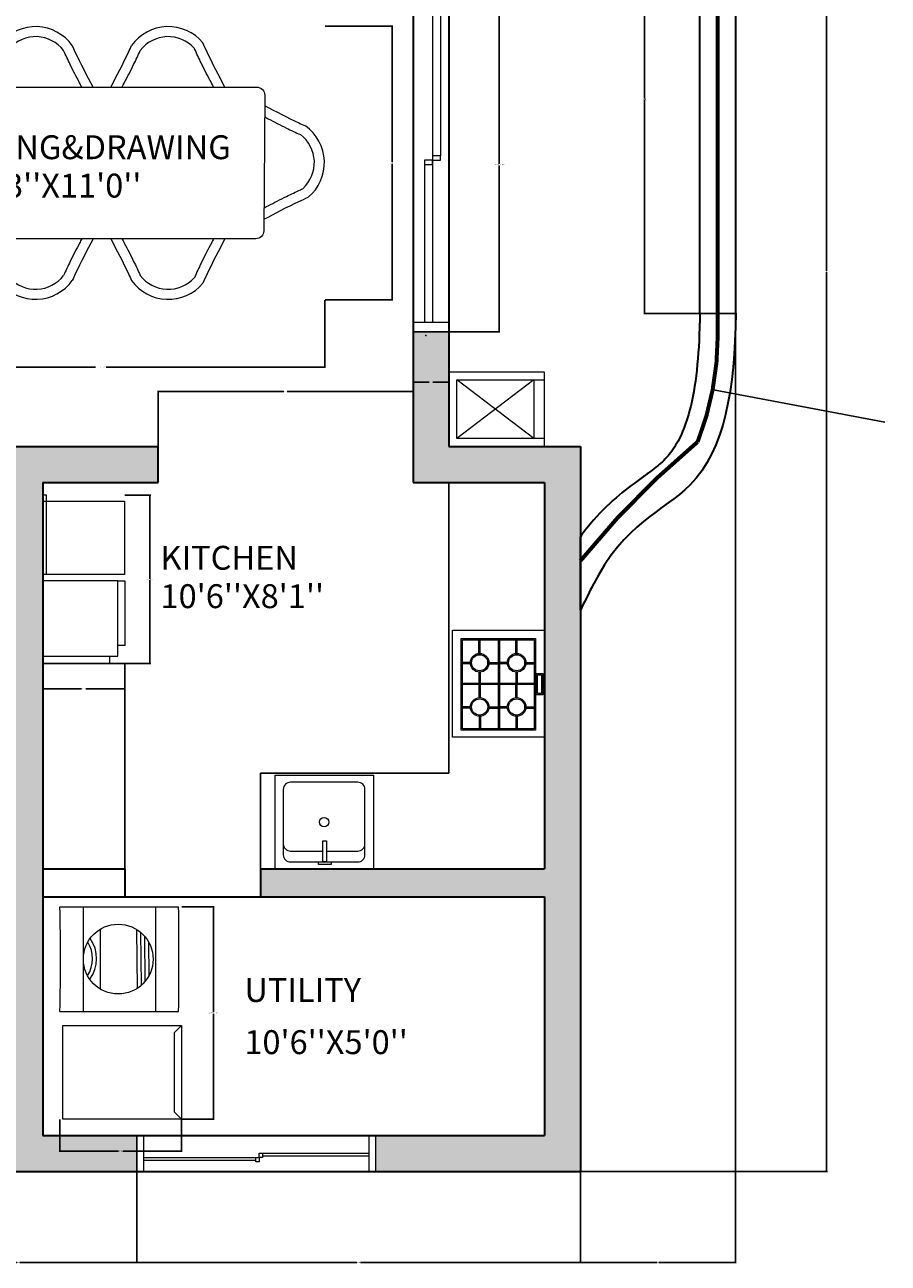
# Model space of a CAD drawing. Units: inches. Extents: x 1789 to 2841, y 3180 to 3702.
# Tile 11 of 14: x 2624 to 2841, y 3180 to 3491. Entities that reach past the tile are written whole.
import ezdxf

# ---------------------------------------------------------------- set-up
doc = ezdxf.new("R2010")
doc.units = ezdxf.units.IN
doc.header["$MEASUREMENT"] = 0
for name, color, linetype, lineweight in [('A-ANNO-DIMS', 2, 'Continuous', 18), ('A-AREA-IDEN', 7, 'Continuous', 18), ('A-EQPM', 8, 'Continuous', 18), ('A-FLOR-CASE', 34, 'Continuous', 25), ('A-FLOR-FIXT', 9, 'Continuous', 18), ('A-FLOR-HRAL', 40, 'Continuous', 18), ('A-WALL', 40, 'Continuous', 35), ('A-WALL-PATT', 252, 'Continuous', 13), ('FURNITURE', 34, 'Continuous', 18), ('WINDOWS', 130, 'Continuous', 18)]:
    doc.layers.add(name, color=color, linetype=linetype, lineweight=lineweight)
doc.styles.get("Standard").update_dxf_attribs({"font": 'arial.ttf'})
doc.dimstyles.get("Standard").update_dxf_attribs({"dimtxt": 0.18, "dimasz": 0.18, "dimexe": 0.18, "dimexo": 0.0625, "dimgap": 0.09, "dimtad": 0, "dimtih": 1, "dimtoh": 1, "dimdec": 0, "dimzin": 0, "dimdsep": 46, "dimlunit": 3, "dimtxsty": 'Standard', "dimcen": 0.09, "dimadec": 0, "dimazin": 0, "dimtfac": 1, "dimtdec": 0, "dimtofl": 0, "dimtmove": 0, "dimatfit": 3, "dimfxl": 1, "dimtolj": 1, "dimtzin": 0, "dimarcsym": 0})

# ---------------------------------------------------------------- blocks, each defined once
blk = doc.blocks.new('WINDOW')
for p, q in [((1997.14, 3495.61), (1997.14, 3458.2)), ((1999.14, 3495.61), (1999.14, 3458.2)), ((1995.14, 3457.08), (1995.14, 3416.32)), ((1997.14, 3457.08), (1997.14, 3416.32))]:
    blk.add_line(p, q)
for points in [[(1992.23, 3497.95), (2001.23, 3497.95), (2001.23, 3413.99), (1992.23, 3413.99)], [(1992.23, 3497.95), (2001.23, 3497.95), (2001.23, 3495.61), (1992.23, 3495.61)], [(1997.14, 3457.08), (1999.14, 3457.08), (1999.14, 3458.2), (1997.14, 3458.2)], [(1995.14, 3455.97), (1997.14, 3455.97), (1997.14, 3457.08), (1995.14, 3457.08)], [(1992.23, 3413.99), (2001.23, 3413.99), (2001.23, 3416.32), (1992.23, 3416.32)]]:
    blk.add_lwpolyline(points, close=True)
blk = doc.blocks.new('HYJ')
for p, q in [((2236.02, 3650.77), (2262.74, 3650.77)), ((2206.12, 3649.67), (2234.3, 3649.67)), ((2206.12, 3649), (2234.3, 3649)), ((2236.02, 3650.11), (2262.74, 3650.11))]:
    blk.add_line(p, q)
for points in [[(2204.43, 3646.16), (2264.43, 3646.16), (2264.43, 3655.16), (2204.43, 3655.16)], [(2204.43, 3655.16), (2206.12, 3655.16), (2206.12, 3646.16), (2204.43, 3646.16)], [(2264.43, 3655.16), (2262.74, 3655.16), (2262.74, 3646.16), (2264.43, 3646.16)], [(2235.16, 3650.77), (2236.02, 3650.77), (2236.02, 3649.67), (2235.16, 3649.67)], [(2234.3, 3649.67), (2235.16, 3649.67), (2235.16, 3648.56), (2234.3, 3648.56)]]:
    blk.add_lwpolyline(points, close=True)
blk = doc.blocks.new('WASH')
for p, q in [((2194.57, 3269.63), (2224.37, 3269.63)), ((2200.44, 3243.35), (2200.44, 3269.63)), ((2218.58, 3269.63), (2218.58, 3243.35)), ((2204.7, 3264.01), (2204.68, 3248.99)), ((2213.79, 3263.95), (2213.93, 3249.12)), ((2214.8, 3263.23), (2214.92, 3249.86)), ((2215.81, 3262.24), (2215.91, 3250.86)), ((2216.82, 3260.81), (2216.9, 3252.31)), ((2194.57, 3243.35), (2224.37, 3243.35)), ((2225.07, 3239.8), (2223.31, 3238.03)), ((2223.31, 3218.04), (2223.31, 3238.03)), ((2225.07, 3216.27), (2223.31, 3218.04))]:
    blk.add_line(p, q)
blk.add_lwpolyline([(2195.28, 3239.8), (2225.07, 3239.8), (2225.07, 3216.27), (2195.28, 3216.27)], close=True)
blk.add_circle((2209.2, 3256.49), 8.76)
for centre, radius, start, end in [((1539.89, 3256.49), 654.81, 358.85012, 1.14988), ((1226.25, 3256.49), 998.2, 359.24572, 0.75428), ((2194.95, 3256.62), 7.81, 326.7676, 32.1994), ((2194.95, 3256.62), 8.81, 323.7828, 35.1842)]:
    blk.add_arc(centre, radius, start, end)
blk = doc.blocks.new('SINK')
for points in [[(2247.56, 3305.33), (2275.07, 3305.33), (2275.07, 3279.16), (2247.56, 3279.16)], [(2260.91, 3287.01), (2261.87, 3287.01), (2261.87, 3281.09), (2260.91, 3281.09)], [(2259.67, 3281.09), (2263.21, 3281.09), (2263.21, 3280.41), (2259.67, 3280.41)]]:
    blk.add_lwpolyline(points, close=True)
blk.add_lwpolyline([(2251.84, 3281.09), (2270.63, 3281.09, 0.414214), (2272.63, 3283.09), (2272.63, 3301.33, 0.414214), (2270.63, 3303.33), (2251.84, 3303.33, 0.414214), (2249.84, 3301.33), (2249.84, 3283.09, 0.414214)], format="xyb", close=True)
for points in [[(2249.84, 3301.33), (2249.84, 3286.11, 0.414214), (2251.84, 3284.11), (2260.91, 3284.11)], [(2261.87, 3284.11), (2270.63, 3284.11, 0.414214), (2272.63, 3286.11), (2272.63, 3301.33)]]:
    blk.add_lwpolyline(points, format="xyb")
blk.add_circle((2261.24, 3292.21), 1.3)
blk = doc.blocks.new('STOVE')
for p, q in [((2291.13, 3337.23), (2291.13, 3342.37)), ((2291.63, 3337.23), (2291.63, 3342.37)), ((2298.52, 3342.42), (2298.52, 3308.4)), ((2299.02, 3342.42), (2299.02, 3308.4)), ((2305.31, 3337.23), (2305.31, 3342.37)), ((2305.81, 3337.23), (2305.81, 3342.37)), ((2287.79, 3333.73), (2284.84, 3333.73)), ((2287.81, 3333.23), (2284.84, 3333.23)), ((2294.92, 3333.23), (2298.52, 3333.23)), ((2294.94, 3333.73), (2298.52, 3333.73)), ((2301.97, 3333.73), (2299.02, 3333.73)), ((2301.99, 3333.23), (2299.02, 3333.23)), ((2309.1, 3333.23), (2312.22, 3333.23)), ((2309.12, 3333.73), (2312.22, 3333.73)), ((2291.13, 3330.09), (2291.13, 3325.91)), ((2291.63, 3330.09), (2291.63, 3325.91)), ((2305.31, 3330.09), (2305.31, 3325.91)), ((2305.81, 3330.09), (2305.81, 3325.91)), ((2284.82, 3325.91), (2312.22, 3325.91)), ((2284.82, 3325.41), (2312.22, 3325.41)), ((2291.15, 3320.29), (2291.15, 3325.43)), ((2291.65, 3320.29), (2291.65, 3325.43)), ((2305.31, 3320.29), (2305.31, 3325.43)), ((2305.31, 3325.41), (2305.31, 3325.34)), ((2305.81, 3320.29), (2305.81, 3325.43)), ((2305.81, 3325.41), (2305.81, 3325.34)), ((2287.8, 3316.79), (2284.82, 3316.79)), ((2287.83, 3316.29), (2284.82, 3316.29)), ((2291.15, 3313.15), (2291.15, 3308.4)), ((2291.65, 3313.15), (2291.65, 3308.4)), ((2294.94, 3316.29), (2298.52, 3316.29)), ((2294.96, 3316.79), (2298.52, 3316.79)), ((2301.97, 3316.79), (2299.02, 3316.79)), ((2301.99, 3316.29), (2299.02, 3316.29)), ((2305.31, 3313.15), (2305.31, 3308.4)), ((2305.81, 3313.15), (2305.81, 3308.4)), ((2309.1, 3316.29), (2312.22, 3316.29)), ((2309.12, 3316.79), (2312.22, 3316.79))]:
    blk.add_line(p, q)
for points in [[(2280.96, 3346.14), (2316.23, 3346.14), (2316.23, 3305.13), (2280.96, 3305.13)], [(2284.32, 3342.92), (2312.72, 3342.92), (2312.72, 3307.9), (2284.32, 3307.9)], [(2284.82, 3342.42), (2312.22, 3342.42), (2312.22, 3308.4), (2284.82, 3308.4)], [(2313.05, 3329.49), (2315.55, 3329.49), (2315.55, 3321.33), (2313.05, 3321.33)], [(2313.55, 3328.99), (2315.05, 3328.99), (2315.05, 3321.83), (2313.55, 3321.83)]]:
    blk.add_lwpolyline(points, close=True)
for centre, radius in [((2291.37, 3333.66), 3.58), ((2291.37, 3333.66), 3.08), ((2305.55, 3333.66), 3.58), ((2305.55, 3333.66), 3.08), ((2291.38, 3316.72), 3.58), ((2291.38, 3316.72), 3.08), ((2305.55, 3316.72), 3.58), ((2305.55, 3316.72), 3.08)]:
    blk.add_circle(centre, radius)
blk = doc.blocks.new('BYY')
for p, q in [((2191.23, 3321.4), (2190.23, 3321.4)), ((2190.23, 3321.4), (2190.23, 3319.89)), ((2191.23, 3301.51), (2191.23, 3321.4)), ((2209.12, 3299.92), (2210.83, 3299.92)), ((2210.83, 3299.92), (2210.83, 3283.66)), ((2190.23, 3279.16), (2190.23, 3281.03)), ((2207.05, 3281.03), (2207.05, 3279.16)), ((2210.83, 3283.66), (2209.12, 3283.66)), ((2207.05, 3279.16), (2190.23, 3279.16))]:
    blk.add_line(p, q)
for points in [[(2190.23, 3319.89), (2210.75, 3319.89), (2210.75, 3301.51), (2190.23, 3301.51)], [(2190.23, 3281.03), (2209.12, 3281.03), (2209.12, 3299.92), (2190.23, 3299.92)]]:
    blk.add_lwpolyline(points, close=True)
blk = doc.blocks.new('DINI')
blk.add_lwpolyline([(2038.22, 3475.42), (2115.97, 3475.42, -0.414214), (2117.97, 3473.42), (2117.72, 3439.35, -0.414214), (2115.72, 3437.35), (2037.97, 3437.35, -0.414214), (2035.97, 3439.35), (2036.22, 3473.42, -0.414214)], format="xyb", close=True)
for centre, radius, start, end in [((2060.43, 3479.31), 11.31, 35.4017, 140.0736), ((2093.76, 3479.31), 11.31, 39.9264, 144.5983), ((2060.43, 3479.31), 8.8, 36.8657, 137.9611), ((2093.76, 3479.31), 8.8, 42.0389, 143.1343), ((2032.05, 3456.46), 11.31, 125.4017, 230.0736), ((2121.64, 3456.46), 11.31, 309.9264, 54.5983), ((2032.05, 3456.46), 8.8, 126.8657, 227.9611), ((2121.64, 3456.46), 8.8, 312.0389, 53.1343), ((2060.43, 3433.45), 11.31, 219.9264, 324.5983), ((2060.43, 3433.45), 8.8, 222.0389, 323.1343), ((2093.76, 3433.45), 11.31, 215.4017, 320.0736), ((2093.76, 3433.45), 8.8, 216.8657, 317.9611)]:
    blk.add_arc(centre, radius, start, end)
for points, knots in [([(2046.22, 3475.42), (2047.75, 3478.33), (2049.68, 3482.01), (2051.4, 3485.79), (2051.76, 3486.58)], [0, 0, 0, 0, 7.856931, 9.915256, 9.915256, 9.915256, 9.915256]), ([(2074.88, 3475.42), (2073.35, 3478.33), (2071.54, 3481.78), (2069.91, 3485.32), (2069.66, 3485.87)], [0, 0, 0, 0, 7.856931, 9.297576, 9.297576, 9.297576, 9.297576]), ([(2079.31, 3475.42), (2080.85, 3478.33), (2082.66, 3481.78), (2084.29, 3485.32), (2084.54, 3485.87)], [0, 0, 0, 0, 7.856931, 9.297576, 9.297576, 9.297576, 9.297576]), ([(2107.98, 3475.42), (2106.45, 3478.33), (2104.51, 3482.01), (2102.79, 3485.79), (2102.44, 3486.58)], [0, 0, 0, 0, 7.856931, 9.915256, 9.915256, 9.915256, 9.915256]), ([(2049.05, 3475.42), (2049.25, 3475.79), (2049.44, 3476.15), (2050.42, 3478.03), (2051.21, 3479.56), (2052.54, 3482.27), (2053.1, 3483.45), (2053.72, 3484.82), (2053.81, 3485.01), (2053.9, 3485.21)], [1.048693, 1.048693, 1.048693, 1.048693, 2.029233, 2.029233, 6.0877, 6.0877, 9.118148, 9.118148, 9.624349, 9.624349, 9.624349, 9.624349]), ([(2072.04, 3475.42), (2071.85, 3475.78), (2071.66, 3476.15), (2070.68, 3478.03), (2069.89, 3479.55), (2068.56, 3482.26), (2068.01, 3483.43), (2067.48, 3484.59)], [1.048889, 1.048889, 1.048889, 1.048889, 2.02655, 2.02655, 6.079649, 6.079649, 9.095857, 9.095857, 9.095857, 9.095857]), ([(2082.15, 3475.42), (2082.34, 3475.78), (2082.53, 3476.15), (2083.51, 3478.03), (2084.3, 3479.55), (2085.63, 3482.26), (2086.19, 3483.43), (2086.72, 3484.59)], [1.048889, 1.048889, 1.048889, 1.048889, 2.02655, 2.02655, 6.079649, 6.079649, 9.095857, 9.095857, 9.095857, 9.095857]), ([(2105.14, 3475.42), (2104.95, 3475.79), (2104.76, 3476.15), (2103.78, 3478.03), (2102.99, 3479.56), (2101.65, 3482.27), (2101.1, 3483.45), (2100.47, 3484.82), (2100.38, 3485.01), (2100.3, 3485.21)], [1.048693, 1.048693, 1.048693, 1.048693, 2.029233, 2.029233, 6.0877, 6.0877, 9.118148, 9.118148, 9.624349, 9.624349, 9.624349, 9.624349]), ([(2036.2, 3471.04), (2036.05, 3470.96), (2035.89, 3470.88), (2035.74, 3470.8), (2035.74, 3470.8), (2035.74, 3470.8), (2035.74, 3470.8), (2032.89, 3469.3), (2029.51, 3467.53), (2026.05, 3465.93), (2025.5, 3465.68)], [-0.229823, -0.229823, -0.229823, -0.229823, 0.189373, 0.189373, 0.189373, 0.189712, 0.189712, 0.189712, 7.856931, 9.297576, 9.297576, 9.297576, 9.297576]), ([(2117.95, 3470.8), (2120.8, 3469.3), (2124.18, 3467.53), (2127.64, 3465.93), (2128.19, 3465.68)], [0.189712, 0.189712, 0.189712, 0.189712, 7.856931, 9.297576, 9.297576, 9.297576, 9.297576]), ([(2036.18, 3468.19), (2036.04, 3468.12), (2035.9, 3468.04), (2035.76, 3467.97), (2035.76, 3467.97), (2035.76, 3467.97), (2035.76, 3467.97), (2035.46, 3467.81), (2035.16, 3467.65), (2033.34, 3466.71), (2031.81, 3465.92), (2029.11, 3464.59), (2027.94, 3464.04), (2026.77, 3463.5)], [0.838882, 0.838882, 0.838882, 0.838882, 1.215073, 1.215073, 1.215073, 1.219193, 1.219193, 1.219193, 2.02655, 2.02655, 6.079649, 6.079649, 9.095857, 9.095857, 9.095857, 9.095857]), ([(2117.93, 3467.97), (2118.23, 3467.81), (2118.53, 3467.65), (2120.35, 3466.71), (2121.88, 3465.92), (2124.58, 3464.59), (2125.75, 3464.04), (2126.92, 3463.5)], [1.219193, 1.219193, 1.219193, 1.219193, 2.02655, 2.02655, 6.079649, 6.079649, 9.095857, 9.095857, 9.095857, 9.095857]), ([(2035.95, 3445.08), (2035.58, 3445.27), (2035.22, 3445.46), (2033.34, 3446.45), (2031.81, 3447.23), (2029.1, 3448.57), (2027.92, 3449.12), (2026.55, 3449.75), (2026.36, 3449.84), (2026.16, 3449.93)], [1.048693, 1.048693, 1.048693, 1.048693, 2.029233, 2.029233, 6.0877, 6.0877, 9.118148, 9.118148, 9.624349, 9.624349, 9.624349, 9.624349]), ([(2117.74, 3445.08), (2118.11, 3445.27), (2118.47, 3445.46), (2120.35, 3446.45), (2121.88, 3447.23), (2124.59, 3448.57), (2125.77, 3449.12), (2127.14, 3449.75), (2127.33, 3449.84), (2127.53, 3449.93)], [1.048693, 1.048693, 1.048693, 1.048693, 2.029233, 2.029233, 6.0877, 6.0877, 9.118148, 9.118148, 9.624349, 9.624349, 9.624349, 9.624349]), ([(2035.95, 3442.24), (2033.03, 3443.77), (2029.36, 3445.71), (2025.58, 3447.43), (2024.79, 3447.79)], [0, 0, 0, 0, 7.856931, 9.915256, 9.915256, 9.915256, 9.915256]), ([(2117.74, 3442.24), (2120.66, 3443.77), (2124.33, 3445.71), (2128.11, 3447.43), (2128.9, 3447.79)], [0, 0, 0, 0, 7.856931, 9.915256, 9.915256, 9.915256, 9.915256]), ([(2046.22, 3437.35), (2047.75, 3434.43), (2049.68, 3430.75), (2051.4, 3426.98), (2051.76, 3426.19)], [0, 0, 0, 0, 7.856931, 9.915256, 9.915256, 9.915256, 9.915256]), ([(2049.05, 3437.35), (2049.25, 3436.98), (2049.44, 3436.62), (2050.42, 3434.73), (2051.21, 3433.2), (2052.54, 3430.5), (2053.1, 3429.32), (2053.72, 3427.95), (2053.81, 3427.75), (2053.9, 3427.56)], [1.048693, 1.048693, 1.048693, 1.048693, 2.029233, 2.029233, 6.0877, 6.0877, 9.118148, 9.118148, 9.624349, 9.624349, 9.624349, 9.624349]), ([(2072.04, 3437.35), (2071.85, 3436.98), (2071.66, 3436.62), (2070.68, 3434.74), (2069.89, 3433.21), (2068.56, 3430.51), (2068.01, 3429.34), (2067.48, 3428.17)], [1.048889, 1.048889, 1.048889, 1.048889, 2.02655, 2.02655, 6.079649, 6.079649, 9.095857, 9.095857, 9.095857, 9.095857]), ([(2074.88, 3437.35), (2073.35, 3434.43), (2071.54, 3430.98), (2069.91, 3427.45), (2069.66, 3426.9)], [0, 0, 0, 0, 7.856931, 9.297576, 9.297576, 9.297576, 9.297576]), ([(2079.31, 3437.35), (2080.85, 3434.43), (2082.66, 3430.98), (2084.29, 3427.45), (2084.54, 3426.9)], [0, 0, 0, 0, 7.856931, 9.297576, 9.297576, 9.297576, 9.297576]), ([(2082.15, 3437.35), (2082.34, 3436.98), (2082.53, 3436.62), (2083.51, 3434.74), (2084.3, 3433.21), (2085.63, 3430.51), (2086.19, 3429.34), (2086.72, 3428.17)], [1.048889, 1.048889, 1.048889, 1.048889, 2.02655, 2.02655, 6.079649, 6.079649, 9.095857, 9.095857, 9.095857, 9.095857]), ([(2105.14, 3437.35), (2104.95, 3436.98), (2104.76, 3436.62), (2103.78, 3434.73), (2102.99, 3433.2), (2101.65, 3430.5), (2101.1, 3429.32), (2100.47, 3427.95), (2100.38, 3427.75), (2100.3, 3427.56)], [1.048693, 1.048693, 1.048693, 1.048693, 2.029233, 2.029233, 6.0877, 6.0877, 9.118148, 9.118148, 9.624349, 9.624349, 9.624349, 9.624349]), ([(2107.98, 3437.35), (2106.45, 3434.43), (2104.51, 3430.75), (2102.79, 3426.98), (2102.44, 3426.19)], [0, 0, 0, 0, 7.856931, 9.915256, 9.915256, 9.915256, 9.915256])]:
    blk.add_open_spline(points, degree=3, knots=knots)
blk = doc.blocks.new('GTGTGTGT')
for p, q in [((1970.85, 3401.93), (1970.85, 3387.16)), ((1970.92, 3401.93), (1990.23, 3387.16)), ((1970.92, 3387.16), (1990.23, 3401.93))]:
    blk.add_line(p, q)
for points in [[(1992.23, 3385.16), (1968.3, 3385.16), (1968.3, 3403.93), (1992.23, 3403.93)], [(1990.23, 3387.16), (1968.3, 3387.16), (1968.3, 3401.93), (1990.23, 3401.93)]]:
    blk.add_lwpolyline(points, close=True)
blk = doc.blocks.new('COUNTER-KITCHEN-L')
for p, q in [((47.28, 97), (47.28, 24)), ((0, 24), (47.28, 24)), ((0, 0), (0, 24))]:
    blk.add_line(p, q)
blk = doc.blocks.new('*D35')
at = {"layer": 'A-ANNO-DIMS', "color": 0, "lineweight": -2, "transparency": 16777216}
for p, q in [((2730.3, 3497.95), (2743.01, 3497.95)), ((2742.83, 3497.77), (2742.83, 3456.15)), ((2742.83, 3414.17), (2742.83, 3455.78)), ((2730.3, 3413.99), (2743.01, 3413.99))]:
    blk.add_line(p, q, dxfattribs=at)
at = {"layer": 'A-ANNO-DIMS', "color": 0, "transparency": 16777216}
for points in [[(2742.8, 3497.77), (2742.86, 3497.77), (2742.83, 3497.95)], [(2742.8, 3414.17), (2742.86, 3414.17), (2742.83, 3413.99)]]:
    blk.add_solid(points, dxfattribs=at)
at = {"layer": 'Defpoints', "color": 0, "transparency": 16777216}
for p in [(2730.23, 3497.95), (2742.83, 3497.95), (2730.23, 3413.99)]:
    blk.add_point(p, dxfattribs=at)
at = {"layer": 'A-ANNO-DIMS', "color": 0, "transparency": 16777216, "insert": (2742.83, 3455.97), "char_height": 0.18, "attachment_point": 5}
blk.add_mtext('\\A1;LIVING WINDOW 84 TYP.', dxfattribs=at)
blk = doc.blocks.new('*D36')
at = {"layer": 'A-ANNO-DIMS', "color": 0, "lineweight": -2, "transparency": 16777216}
for p, q in [((2721.23, 3413.93), (2721.23, 3401.21)), ((2730.23, 3413.93), (2730.23, 3401.21)), ((2721.41, 3401.39), (2725.28, 3401.39)), ((2730.05, 3401.39), (2726.19, 3401.39))]:
    blk.add_line(p, q, dxfattribs=at)
at = {"layer": 'A-ANNO-DIMS', "color": 0, "transparency": 16777216}
for points in [[(2721.41, 3401.42), (2721.41, 3401.36), (2721.23, 3401.39)], [(2730.05, 3401.42), (2730.05, 3401.36), (2730.23, 3401.39)]]:
    blk.add_solid(points, dxfattribs=at)
at = {"layer": 'Defpoints', "color": 0, "transparency": 16777216}
for p in [(2721.23, 3413.99), (2730.23, 3413.99), (2730.23, 3401.39)]:
    blk.add_point(p, dxfattribs=at)
at = {"layer": 'A-ANNO-DIMS', "color": 0, "transparency": 16777216, "insert": (2725.73, 3401.39), "char_height": 0.18, "attachment_point": 5}
blk.add_mtext('\\A1;9 TYP.', dxfattribs=at)
blk = doc.blocks.new('*D61')
at = {"layer": 'A-ANNO-DIMS', "color": 0, "lineweight": -2, "transparency": 16777216}
for p, q in [((2663.14, 3269.63), (2671.26, 3269.63)), ((2671.08, 3269.45), (2671.08, 3243.14)), ((2671.08, 3216.45), (2671.08, 3242.77)), ((2663.14, 3216.27), (2671.26, 3216.27))]:
    blk.add_line(p, q, dxfattribs=at)
at = {"layer": 'A-ANNO-DIMS', "color": 0, "transparency": 16777216}
for points in [[(2671.05, 3269.45), (2671.11, 3269.45), (2671.08, 3269.63)], [(2671.05, 3216.45), (2671.11, 3216.45), (2671.08, 3216.27)]]:
    blk.add_solid(points, dxfattribs=at)
at = {"layer": 'Defpoints', "color": 0, "transparency": 16777216}
for p in [(2663.07, 3269.63), (2671.08, 3269.63), (2663.07, 3216.27)]:
    blk.add_point(p, dxfattribs=at)
at = {"layer": 'A-ANNO-DIMS', "color": 0, "transparency": 16777216, "insert": (2671.08, 3242.95), "char_height": 0.18, "attachment_point": 5}
blk.add_mtext('\\A1;LAUNDRY UNIT 53 TYP.', dxfattribs=at)
blk = doc.blocks.new('*D62')
at = {"layer": 'A-ANNO-DIMS', "color": 0, "lineweight": -2, "transparency": 16777216}
for p, q in [((2632.57, 3216.21), (2632.57, 3208.09)), ((2663.07, 3216.21), (2663.07, 3208.09)), ((2632.75, 3208.27), (2647.29, 3208.27)), ((2662.89, 3208.27), (2648.35, 3208.27))]:
    blk.add_line(p, q, dxfattribs=at)
at = {"layer": 'A-ANNO-DIMS', "color": 0, "transparency": 16777216}
for points in [[(2632.75, 3208.3), (2632.75, 3208.24), (2632.57, 3208.27)], [(2662.89, 3208.3), (2662.89, 3208.24), (2663.07, 3208.27)]]:
    blk.add_solid(points, dxfattribs=at)
at = {"layer": 'Defpoints', "color": 0, "transparency": 16777216}
for p in [(2632.57, 3216.27), (2663.07, 3216.27), (2663.07, 3208.27)]:
    blk.add_point(p, dxfattribs=at)
at = {"layer": 'A-ANNO-DIMS', "color": 0, "transparency": 16777216, "insert": (2647.82, 3208.27), "char_height": 0.18, "attachment_point": 5}
blk.add_mtext('\\A1;31 TYP.', dxfattribs=at)
blk = doc.blocks.new('*D65')
at = {"layer": 'A-ANNO-DIMS', "color": 0, "lineweight": -2, "transparency": 16777216}
for p, q in [((2648.89, 3372.95), (2655.35, 3372.95)), ((2655.17, 3372.77), (2655.17, 3352.01)), ((2655.17, 3330.88), (2655.17, 3351.64)), ((2648.89, 3330.7), (2655.35, 3330.7))]:
    blk.add_line(p, q, dxfattribs=at)
at = {"layer": 'A-ANNO-DIMS', "color": 0, "transparency": 16777216}
for points in [[(2655.14, 3372.77), (2655.2, 3372.77), (2655.17, 3372.95)], [(2655.14, 3330.88), (2655.2, 3330.88), (2655.17, 3330.7)]]:
    blk.add_solid(points, dxfattribs=at)
at = {"layer": 'Defpoints', "color": 0, "transparency": 16777216}
for p in [(2648.83, 3372.95), (2655.17, 3372.95), (2648.83, 3330.7)]:
    blk.add_point(p, dxfattribs=at)
at = {"layer": 'A-ANNO-DIMS', "color": 0, "transparency": 16777216, "insert": (2655.17, 3351.83), "char_height": 0.18, "attachment_point": 5}
blk.add_mtext('\\A1;KITCHEN UNIT 42 TYP.', dxfattribs=at)
blk = doc.blocks.new('*D66')
at = {"layer": 'A-ANNO-DIMS', "color": 0, "lineweight": -2, "transparency": 16777216}
for p, q in [((2628.23, 3330.64), (2628.23, 3324.19)), ((2648.83, 3330.64), (2648.83, 3324.19)), ((2628.41, 3324.37), (2638, 3324.37)), ((2648.65, 3324.37), (2639.06, 3324.37))]:
    blk.add_line(p, q, dxfattribs=at)
at = {"layer": 'A-ANNO-DIMS', "color": 0, "transparency": 16777216}
for points in [[(2628.41, 3324.4), (2628.41, 3324.34), (2628.23, 3324.37)], [(2648.65, 3324.4), (2648.65, 3324.34), (2648.83, 3324.37)]]:
    blk.add_solid(points, dxfattribs=at)
at = {"layer": 'Defpoints', "color": 0, "transparency": 16777216}
for p in [(2628.23, 3330.7), (2648.83, 3330.7), (2648.83, 3324.37)]:
    blk.add_point(p, dxfattribs=at)
at = {"layer": 'A-ANNO-DIMS', "color": 0, "transparency": 16777216, "insert": (2638.53, 3324.37), "char_height": 0.18, "attachment_point": 5}
blk.add_mtext('\\A1;21 TYP.', dxfattribs=at)
blk = doc.blocks.new('*D71')
at = {"layer": 'A-ANNO-DIMS', "color": 0, "lineweight": -2, "transparency": 16777216}
for p, q in [((2586.62, 3421.95), (2586.62, 3404.96)), ((2699.09, 3421.95), (2699.09, 3404.96)), ((2586.8, 3405.14), (2641.51, 3405.14)), ((2698.91, 3405.14), (2644.2, 3405.14))]:
    blk.add_line(p, q, dxfattribs=at)
at = {"layer": 'A-ANNO-DIMS', "color": 0, "transparency": 16777216}
for points in [[(2586.8, 3405.17), (2586.8, 3405.11), (2586.62, 3405.14)], [(2698.91, 3405.17), (2698.91, 3405.11), (2699.09, 3405.14)]]:
    blk.add_solid(points, dxfattribs=at)
at = {"layer": 'Defpoints', "color": 0, "transparency": 16777216}
for p in [(2586.62, 3422.01), (2699.09, 3422.01), (2699.09, 3405.14)]:
    blk.add_point(p, dxfattribs=at)
at = {"layer": 'A-ANNO-DIMS', "color": 0, "transparency": 16777216, "insert": (2642.85, 3405.14), "char_height": 0.18, "attachment_point": 5}
blk.add_mtext('\\A1;DINING SET 112 TYP.', dxfattribs=at)
blk = doc.blocks.new('*D72')
at = {"layer": 'A-ANNO-DIMS', "color": 0, "lineweight": -2, "transparency": 16777216}
for p, q in [((2699.15, 3490.76), (2716.14, 3490.76)), ((2715.96, 3490.58), (2715.96, 3456.57)), ((2715.96, 3422.19), (2715.96, 3456.2)), ((2699.15, 3422.01), (2716.14, 3422.01))]:
    blk.add_line(p, q, dxfattribs=at)
at = {"layer": 'A-ANNO-DIMS', "color": 0, "transparency": 16777216}
for points in [[(2715.93, 3490.58), (2715.99, 3490.58), (2715.96, 3490.76)], [(2715.93, 3422.19), (2715.99, 3422.19), (2715.96, 3422.01)]]:
    blk.add_solid(points, dxfattribs=at)
at = {"layer": 'Defpoints', "color": 0, "transparency": 16777216}
for p in [(2699.09, 3490.76), (2715.96, 3490.76), (2699.09, 3422.01)]:
    blk.add_point(p, dxfattribs=at)
at = {"layer": 'A-ANNO-DIMS', "color": 0, "transparency": 16777216, "insert": (2715.96, 3456.38), "char_height": 0.18, "attachment_point": 5}
blk.add_mtext('\\A1;69 TYP.', dxfattribs=at)
blk = doc.blocks.new('*D96')
at = {"layer": 'A-ANNO-DIMS', "color": 0, "lineweight": -2, "transparency": 16777216}
for p, q in [((2763.3, 3655.16), (2825.26, 3655.16)), ((2825.08, 3654.98), (2825.08, 3429.34)), ((2825.08, 3203.34), (2825.08, 3428.98)), ((2763.3, 3203.16), (2825.26, 3203.16))]:
    blk.add_line(p, q, dxfattribs=at)
at = {"layer": 'A-ANNO-DIMS', "color": 0, "transparency": 16777216}
for points in [[(2825.05, 3654.98), (2825.11, 3654.98), (2825.08, 3655.16)], [(2825.05, 3203.34), (2825.11, 3203.34), (2825.08, 3203.16)]]:
    blk.add_solid(points, dxfattribs=at)
at = {"layer": 'Defpoints', "color": 0, "transparency": 16777216}
for p in [(2763.23, 3655.16), (2763.23, 3203.16), (2825.08, 3203.16)]:
    blk.add_point(p, dxfattribs=at)
at = {"layer": 'A-ANNO-DIMS', "color": 0, "transparency": 16777216, "insert": (2825.08, 3429.16), "char_height": 0.18, "attachment_point": 5}
blk.add_mtext('\\A1;452', dxfattribs=at)
blk = doc.blocks.new('*D99')
at = {"layer": 'A-ANNO-DIMS', "color": 0, "lineweight": -2, "transparency": 16777216}
for p, q in [((2592.37, 3203.1), (2592.37, 3180.13)), ((2651.85, 3203.1), (2651.85, 3180.13)), ((2592.55, 3180.31), (2621.72, 3180.31)), ((2651.67, 3180.31), (2622.5, 3180.31))]:
    blk.add_line(p, q, dxfattribs=at)
at = {"layer": 'A-ANNO-DIMS', "color": 0, "transparency": 16777216}
for points in [[(2592.55, 3180.34), (2592.55, 3180.28), (2592.37, 3180.31)], [(2651.67, 3180.34), (2651.67, 3180.28), (2651.85, 3180.31)]]:
    blk.add_solid(points, dxfattribs=at)
at = {"layer": 'Defpoints', "color": 0, "transparency": 16777216}
for p in [(2592.37, 3203.16), (2651.85, 3203.16), (2651.85, 3180.31)]:
    blk.add_point(p, dxfattribs=at)
at = {"layer": 'A-ANNO-DIMS', "color": 0, "transparency": 16777216, "insert": (2622.11, 3180.31), "char_height": 0.18, "attachment_point": 5}
blk.add_mtext('\\A1;59.48', dxfattribs=at)
blk = doc.blocks.new('*D100')
at = {"layer": 'A-ANNO-DIMS', "color": 0, "lineweight": -2, "transparency": 16777216}
for p, q in [((2651.85, 3203.1), (2651.85, 3180.13)), ((2763.23, 3203.1), (2763.23, 3180.13)), ((2652.03, 3180.31), (2707.09, 3180.31)), ((2763.05, 3180.31), (2708, 3180.31))]:
    blk.add_line(p, q, dxfattribs=at)
at = {"layer": 'A-ANNO-DIMS', "color": 0, "transparency": 16777216}
for points in [[(2652.03, 3180.34), (2652.03, 3180.28), (2651.85, 3180.31)], [(2763.05, 3180.34), (2763.05, 3180.28), (2763.23, 3180.31)]]:
    blk.add_solid(points, dxfattribs=at)
at = {"layer": 'Defpoints', "color": 0, "transparency": 16777216}
for p in [(2651.85, 3203.16), (2763.23, 3203.16), (2763.23, 3180.31)]:
    blk.add_point(p, dxfattribs=at)
at = {"layer": 'A-ANNO-DIMS', "color": 0, "transparency": 16777216, "insert": (2707.54, 3180.31), "char_height": 0.18, "attachment_point": 5}
blk.add_mtext('\\A1;111.38', dxfattribs=at)
blk = doc.blocks.new('*D101')
at = {"layer": 'A-ANNO-DIMS', "color": 0, "lineweight": -2, "transparency": 16777216}
for p, q in [((2802.23, 3418.57), (2802.23, 3180.13)), ((2763.23, 3203.1), (2763.23, 3180.13)), ((2763.41, 3180.31), (2782.51, 3180.31)), ((2802.05, 3180.31), (2782.95, 3180.31))]:
    blk.add_line(p, q, dxfattribs=at)
at = {"layer": 'A-ANNO-DIMS', "color": 0, "transparency": 16777216}
for points in [[(2763.41, 3180.34), (2763.41, 3180.28), (2763.23, 3180.31)], [(2802.05, 3180.34), (2802.05, 3180.28), (2802.23, 3180.31)]]:
    blk.add_solid(points, dxfattribs=at)
at = {"layer": 'Defpoints', "color": 0, "transparency": 16777216}
for p in [(2802.23, 3418.63), (2763.23, 3203.16), (2802.23, 3180.31)]:
    blk.add_point(p, dxfattribs=at)
at = {"layer": 'A-ANNO-DIMS', "color": 0, "transparency": 16777216, "insert": (2782.73, 3180.31), "char_height": 0.18, "attachment_point": 5}
blk.add_mtext('\\A1;39', dxfattribs=at)
blk = doc.blocks.new('*D112')
at = {"layer": 'A-ANNO-DIMS', "color": 0, "lineweight": -2, "transparency": 16777216}
for p, q in [((2657.2, 3376.22), (2657.2, 3399.19)), ((2657.38, 3399.01), (2688.82, 3399.01)), ((2721.05, 3399.01), (2689.61, 3399.01)), ((2721.23, 3376.22), (2721.23, 3399.19))]:
    blk.add_line(p, q, dxfattribs=at)
at = {"layer": 'A-ANNO-DIMS', "color": 0, "transparency": 16777216}
for points in [[(2657.38, 3399.04), (2657.38, 3398.98), (2657.2, 3399.01)], [(2721.05, 3399.04), (2721.05, 3398.98), (2721.23, 3399.01)]]:
    blk.add_solid(points, dxfattribs=at)
at = {"layer": 'Defpoints', "color": 0, "transparency": 16777216}
for p in [(2721.23, 3399.01), (2657.2, 3376.16), (2721.23, 3376.16)]:
    blk.add_point(p, dxfattribs=at)
at = {"layer": 'A-ANNO-DIMS', "color": 0, "transparency": 16777216, "insert": (2689.22, 3399.01), "char_height": 0.18, "attachment_point": 5}
blk.add_mtext('\\A1;64.04', dxfattribs=at)
blk = doc.blocks.new('*D114')
at = {"layer": 'A-ANNO-DIMS', "color": 0, "lineweight": -2, "transparency": 16777216}
for p, q in [((2802.17, 3526.16), (2779.2, 3526.16)), ((2779.38, 3525.98), (2779.38, 3472.58)), ((2779.38, 3418.81), (2779.38, 3472.21)), ((2802.17, 3418.63), (2779.2, 3418.63))]:
    blk.add_line(p, q, dxfattribs=at)
at = {"layer": 'A-ANNO-DIMS', "color": 0, "transparency": 16777216}
for points in [[(2779.35, 3525.98), (2779.41, 3525.98), (2779.38, 3526.16)], [(2779.35, 3418.81), (2779.41, 3418.81), (2779.38, 3418.63)]]:
    blk.add_solid(points, dxfattribs=at)
at = {"layer": 'Defpoints', "color": 0, "transparency": 16777216}
for p in [(2779.38, 3526.16), (2802.23, 3526.16), (2802.23, 3418.63)]:
    blk.add_point(p, dxfattribs=at)
at = {"layer": 'A-ANNO-DIMS', "color": 0, "transparency": 16777216, "insert": (2779.38, 3472.4), "char_height": 0.18, "attachment_point": 5}
blk.add_mtext('\\A1;107.53', dxfattribs=at)
blk = doc.blocks.new('*D120')
at = {"layer": 'A-ANNO-DIMS', "color": 0, "lineweight": -2, "transparency": 16777216}
for p, q in [((2724.35, 3413.08), (2724.53, 3413.08)), ((2724.44, 3412.99), (2724.44, 3413.17)), ((2839.67, 3391.34), (2796.64, 3399.46))]:
    blk.add_line(p, q, dxfattribs=at)
at = {"layer": 'A-ANNO-DIMS', "color": 0, "transparency": 16777216}
blk.add_solid([(2796.65, 3399.49), (2796.63, 3399.43), (2796.46, 3399.49)], dxfattribs=at)
at = {"layer": 'Defpoints', "color": 0, "transparency": 16777216}
for p in [(2724.44, 3413.08), (2796.46, 3399.49)]:
    blk.add_point(p, dxfattribs=at)
at = {"layer": 'A-ANNO-DIMS', "color": 0, "transparency": 16777216, "insert": (2840.15, 3391.34), "char_height": 0.18, "attachment_point": 5}
blk.add_mtext('\\A1;R73.29', dxfattribs=at)

msp = doc.modelspace()

# ---------------------------------------------------------------- hatches: boundary and pattern name
at = {"layer": 'A-WALL-PATT'}
h = msp.add_hatch(color=256, dxfattribs=at)
h.dxf.hatch_style = 1
h.paths.add_polyline_path([(2763.2333, 3385.1608), (2730.2333, 3385.1608), (2730.2333, 3403.9339), (2730.2333, 3413.9882), (2721.2333, 3413.9882), (2721.2333, 3376.1608), (2754.2333, 3376.1608), (2754.2333, 3279.1608), (2682.9532, 3279.1608), (2682.9532, 3272.1608), (2754.2333, 3272.1608), (2754.2333, 3212.1608), (2711.8514, 3212.1608), (2711.8514, 3203.1608), (2763.2333, 3203.1608), (2763.2333, 3344.1082), (2763.2333, 3362.5259)])
h = msp.add_hatch(color=256, dxfattribs=at)
h.dxf.hatch_style = 1
h.paths.add_polyline_path([(2628.2333, 3376.1608), (2657.1973, 3376.1608), (2657.1973, 3385.1608), (2619.2333, 3385.1608), (2619.2333, 3212.1608), (2616.3707, 3212.1608), (2616.3707, 3203.1608), (2651.8514, 3203.1608), (2651.8514, 3212.1608), (2628.2333, 3212.1608)])

# ---------------------------------------------------------------- linework, layer by layer
at = {"layer": 'A-FLOR-CASE'}
msp.add_lwpolyline([(2628.2333, 3330.704), (2648.8305, 3330.704), (2648.8305, 3272.1608), (2628.2333, 3272.1608)], close=True, dxfattribs=at)
at = {"layer": 'A-FLOR-HRAL', "const_width": 1}
msp.add_lwpolyline([(2763.2333, 3521.6608), (2797.7333, 3521.6608), (2797.7333, 3413.0793, -0.09351003), (2792.6951, 3386.3751, 0.04972233), (2763.2333, 3356.4636)], format="xyb", dxfattribs=at)
at = {"layer": 'A-WALL'}
for p, q in [((2802.2333, 3418.6331), (2802.2333, 3526.1608)), ((2721.2333, 3517.1608), (2721.2333, 3376.1608)), ((2730.2333, 3517.1608), (2730.2333, 3385.1608)), ((2793.2333, 3418.6846), (2793.2333, 3517.1608)), ((2619.2333, 3385.1608), (2657.1973, 3385.1608)), ((2657.1973, 3376.1608), (2657.1973, 3385.1608)), ((2730.2333, 3385.1608), (2763.2333, 3385.1608)), ((2763.2333, 3385.1608), (2763.2333, 3362.5259)), ((2628.2333, 3376.1608), (2628.2333, 3212.1608)), ((2628.2333, 3376.1608), (2657.1973, 3376.1608)), ((2721.2333, 3376.1608), (2754.2333, 3376.1608)), ((2754.2333, 3376.1608), (2754.2333, 3279.1608)), ((2763.2333, 3344.1082), (2763.2333, 3362.5259)), ((2763.2333, 3362.5259), (2763.2333, 3344.1082)), ((2763.2333, 3344.1082), (2763.2333, 3203.1608)), ((2628.2333, 3279.1608), (2648.8305, 3279.1608)), ((2648.8305, 3279.1608), (2648.8305, 3272.1608)), ((2682.9532, 3279.1608), (2754.2333, 3279.1608)), ((2682.9532, 3279.1608), (2682.9532, 3272.1608)), ((2628.2333, 3272.1608), (2754.2333, 3272.1608)), ((2754.2333, 3272.1608), (2754.2333, 3212.1608)), ((2628.2333, 3212.1608), (2754.2333, 3212.1608)), ((2397.2333, 3203.1608), (2763.2333, 3203.1608))]:
    msp.add_line(p, q, dxfattribs=at)
for points, knots in [([(2793.2333, 3418.6846), (2793.2196, 3417.4316), (2793.1954, 3416.1996), (2793.0316, 3410.6781), (2792.7546, 3406.6502), (2791.8315, 3399.3091), (2791.1838, 3395.9979), (2789.7655, 3391.1002), (2789.091, 3389.2951), (2787.5886, 3386.1256), (2786.7629, 3384.7623), (2785.4764, 3383.0786), (2785.0713, 3382.6024), (2784.4248, 3381.9198), (2784.1975, 3381.6934), (2783.6995, 3381.2247), (2783.4322, 3380.9856), (2782.5699, 3380.2487), (2781.9141, 3379.7316), (2780.4391, 3378.6225), (2779.6203, 3378.0307), (2777.0316, 3376.1573), (2775.0725, 3374.7389), (2770.9025, 3371.2603), (2768.6965, 3369.1962), (2765.4122, 3365.4222), (2764.3117, 3364.0358), (2763.2333, 3362.5259)], [4.38907139, 4.38907139, 4.38907139, 4.38907139, 7.6358486, 7.6358486, 19.20888675, 19.20888675, 30.78192491, 30.78192491, 38.89033862, 38.89033862, 46.99875233, 46.99875233, 50.54541348, 50.54541348, 52.44307722, 52.44307722, 54.34074096, 54.34074096, 58.13606845, 58.13606845, 61.93139593, 61.93139593, 69.18500608, 69.18500608, 76.43861623, 76.43861623, 80.13503858, 80.13503858, 80.13503858, 80.13503858]), ([(2802.2333, 3418.6331), (2802.0303, 3399.7176), (2797.6465, 3372.8971), (2774.2891, 3366.077), (2766.2333, 3350.0781), (2766.2181, 3350.0478), (2766.2028, 3350.0174), (2766.1876, 3349.9871), (2765.2028, 3348.0275), (2764.2181, 3346.0678), (2763.2333, 3344.1082)], [4.35013907, 4.35013907, 4.35013907, 4.35013907, 51.40968685, 86.1489403, 86.1489403, 86.1489403, 86.21473832, 86.21473832, 86.21473832, 90.46318188, 90.46318188, 90.46318188, 90.46318188])]:
    msp.add_open_spline(points, degree=3, knots=knots, dxfattribs=at)

# ---------------------------------------------------------------- block references
at = {"layer": 'A-EQPM'}
for name, p in [('BYY', (438, 51.5432)), ('WASH', (438, 0))]:
    msp.add_blockref(name, p, dxfattribs=at)
at = {"layer": 'A-EQPM', "xscale": 0.6553007250005952, "yscale": 0.6553007250005952, "zscale": 0.6553007250005952}
msp.add_blockref('STOVE', (1236.404, 1146.3444), dxfattribs=at)
at = {"layer": 'A-FLOR-CASE'}
msp.add_blockref('COUNTER-KITCHEN-L', (2682.953, 3279.161), dxfattribs=at)
at = {"layer": 'A-FLOR-FIXT', "xscale": 0.8998033160254596, "yscale": 0.8998033160254596, "zscale": 0.8998033160254596}
msp.add_blockref('SINK', (664.22, 328.561), dxfattribs=at)
at = {"layer": 'FURNITURE'}
msp.add_blockref('DINI', (566.0099, 0), dxfattribs=at)
at = {"layer": 'FURNITURE', "rotation": 180}
msp.add_blockref('GTGTGTGT', (4722.4667, 6789.0947), dxfattribs=at)
at = {"layer": 'WINDOWS'}
for name, p in [('WINDOW', (729, 0)), ('HYJ', (447.4189, -443))]:
    msp.add_blockref(name, p, dxfattribs=at)

# ---------------------------------------------------------------- texts
at = {"layer": 'A-ANNO-DIMS'}
for s, p in [("26'3''X11'0''", (2607.4196, 3447.6999)), ("10'6''X8'1''", (2657.8164, 3344.6141)), ("10'6''X5'0''", (2678.8634, 3232.6388))]:
    msp.add_text(s, height=6, dxfattribs=at).set_placement(p)
at = {"layer": 'A-AREA-IDEN'}
for s, p in [('LIVING&DRAWING', (2607.4196, 3457.3383)), ('KITCHEN', (2657.8164, 3354.2526)), ('UTILITY', (2678.8634, 3245.7371))]:
    msp.add_text(s, height=6, dxfattribs=at).set_placement(p)

# ---------------------------------------------------------------- dimensions: what is measured, and where the dimension line sits
at = {"layer": 'A-ANNO-DIMS'}
for base, p1, p2, override, picture, middle in [((2825.0833, 3203.1608), (2763.2333, 3655.1608), (2763.2333, 3203.1608), {"dimdec": 0, "dimlfac": 1, "dimrnd": 0, "dimzin": 0, "dimdsep": 46, "dimlunit": 2}, '*D96', (2825.0833, 3429.1608)), ((2779.3833, 3526.1608), (2802.2333, 3418.6331), (2802.2333, 3526.1608), {"dimdec": 2, "dimlfac": 1, "dimrnd": 0, "dimzin": 0, "dimdsep": 46, "dimlunit": 2}, '*D114', (2779.3833, 3472.3969))]:
    dim = msp.add_linear_dim(base=base, p1=p1, p2=p2, angle=90, dimstyle='Standard', override=override, dxfattribs=at)
    dim.commit()
    dim.dimension.update_dxf_attribs({"geometry": picture, "text_midpoint": middle})
for base, p1, p2, text, picture, middle in [((2742.8271, 3497.9466), (2730.2333, 3413.9882), (2730.2333, 3497.9466), 'LIVING WINDOW <> TYP.', '*D35', (2742.8271, 3455.9674)), ((2715.959, 3490.7571), (2699.0888, 3422.0092), (2699.0888, 3490.7571), '<> TYP.', '*D72', (2715.959, 3456.3832)), ((2655.1669, 3372.9462), (2648.8305, 3330.704), (2648.8305, 3372.9462), 'KITCHEN UNIT <> TYP.', '*D65', (2655.1669, 3351.8251)), ((2671.0773, 3269.6329), (2663.0735, 3216.274), (2663.0735, 3269.6329), 'LAUNDRY UNIT <> TYP.', '*D61', (2671.0773, 3242.9535))]:
    dim = msp.add_linear_dim(base=base, p1=p1, p2=p2, angle=90, text=text, dimstyle='Standard', override={"dimdec": 0, "dimlfac": 1, "dimrnd": 0, "dimzin": 0, "dimdsep": 46, "dimlunit": 2}, dxfattribs=at)
    dim.commit()
    dim.dimension.update_dxf_attribs({"geometry": picture, "text_midpoint": middle})
for base, p1, p2, text, picture, middle in [((2699.0888, 3405.1391), (2586.621, 3422.0092), (2699.0888, 3422.0092), 'DINING SET <> TYP.', '*D71', (2642.8549, 3405.1391)), ((2730.2333, 3401.3945), (2721.2333, 3413.9882), (2730.2333, 3413.9882), '<> TYP.', '*D36', (2725.7333, 3401.3945)), ((2648.8305, 3324.3676), (2628.2333, 3330.704), (2648.8305, 3330.704), '<> TYP.', '*D66', (2638.5319, 3324.3676)), ((2663.0735, 3208.2702), (2632.5709, 3216.274), (2663.0735, 3216.274), '<> TYP.', '*D62', (2647.8222, 3208.2702))]:
    dim = msp.add_linear_dim(base=base, p1=p1, p2=p2, text=text, dimstyle='Standard', override={"dimdec": 0, "dimlfac": 1, "dimrnd": 0, "dimzin": 0, "dimdsep": 46, "dimlunit": 2}, dxfattribs=at)
    dim.commit()
    dim.dimension.update_dxf_attribs({"geometry": picture, "text_midpoint": middle})
for base, p1, p2, override, picture, middle in [((2802.2333, 3180.3108), (2763.2333, 3203.1608), (2802.2333, 3418.6331), {"dimdec": 0, "dimlfac": 1, "dimrnd": 0, "dimzin": 0, "dimdsep": 46, "dimlunit": 2}, '*D101', (2782.7333, 3180.3108)), ((2721.2333, 3399.0108), (2657.1973, 3376.1608), (2721.2333, 3376.1608), {"dimdec": 2, "dimlfac": 1, "dimrnd": 0, "dimzin": 0, "dimdsep": 46, "dimlunit": 2}, '*D112', (2689.2153, 3399.0108)), ((2651.8514, 3180.3108), (2592.3707, 3203.1608), (2651.8514, 3203.1608), {"dimdec": 2, "dimlfac": 1, "dimrnd": 0, "dimzin": 0, "dimdsep": 46, "dimlunit": 2}, '*D99', (2622.1111, 3180.3108)), ((2763.2333, 3180.3108), (2651.8514, 3203.1608), (2763.2333, 3203.1608), {"dimdec": 2, "dimlfac": 1, "dimrnd": 0, "dimzin": 0, "dimdsep": 46, "dimlunit": 2}, '*D100', (2707.5424, 3180.3108))]:
    dim = msp.add_linear_dim(base=base, p1=p1, p2=p2, dimstyle='Standard', override=override, dxfattribs=at)
    dim.commit()
    dim.dimension.update_dxf_attribs({"geometry": picture, "text_midpoint": middle})
dim = msp.add_radius_dim(center=(2724.4444, 3413.0793), mpoint=(2796.4628, 3399.492), dimstyle='Standard', override={"dimdec": 2, "dimlfac": 1, "dimrnd": 0, "dimzin": 0, "dimdsep": 46, "dimlunit": 2}, dxfattribs=at)
dim.commit()
dim.dimension.update_dxf_attribs({"geometry": '*D120', "text_midpoint": (2839.6739, 3391.3397), "dimtype": 164})

doc.saveas('drawing.dxf')
